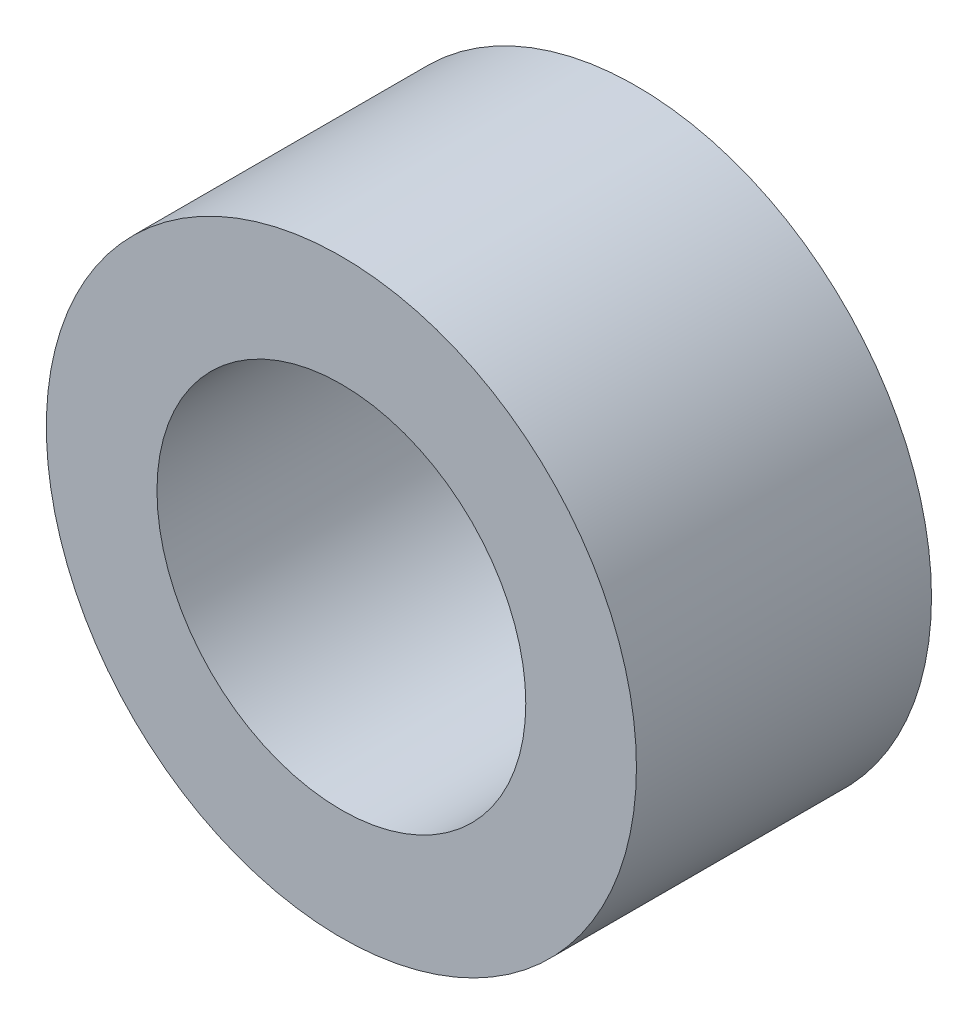
from build123d import *

# Parameters (mm, degrees)
BUSH_RING_PROFILE_10_X_6_25_R   = 5
BUSH_RING_PROFILE_10_X_6_25_R_2 = 3.125
BUSH_BODY_L5_DEPTH              = 2.5


with BuildPart() as part:
    # Bush Ring Profile Ø10 x Ø6.25 → Bush Body L5 (new, symmetric)
    with BuildSketch(Plane.XY):
        Circle(BUSH_RING_PROFILE_10_X_6_25_R)
        Circle(BUSH_RING_PROFILE_10_X_6_25_R_2, mode=Mode.SUBTRACT)
    extrude(amount=BUSH_BODY_L5_DEPTH, both=True)


solid = part.part
